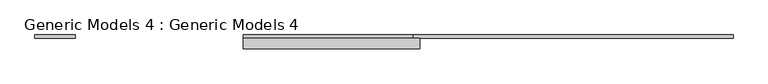
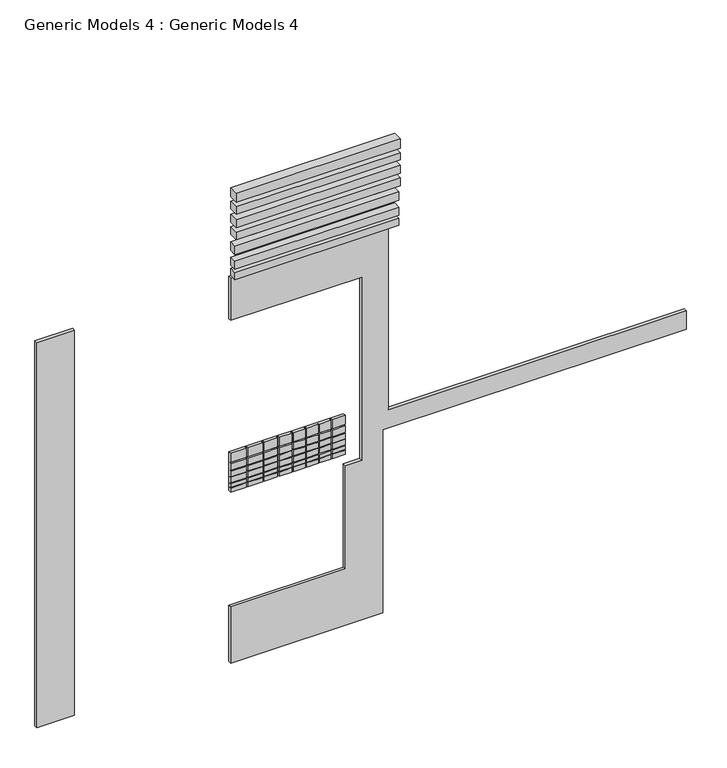
"""IFC4 building model written with IfcOpenShell, lengths in millimetres: proxy geometry, Generic Models 4 : Generic Models 4."""

from ifc_helpers import new_model, si_unit, frame, origin, origin_with_axes, place, context, project, spatial, polyline, outline, extrude, faceted_brep, source, transform, mapped, element, save


def generic_models_4_generic_models_4_7ccdd1b4(model_context):
    return source(origin(), model_context, "Body", "SolidModel", [
        faceted_brep([(-14590.3624893, -13038.0040375, 3489.9238444), (-14590.3624893, -13038.0040375, 3343.084444), (-14347.53389, -13038.0040375, 3343.084444), (-14347.53389, -13038.0040375, 3489.9238444), (-14590.3624893, -13038.0040375, 3318.5039332), (-14590.3624893, -13038.0040375, 3211.3169884), (-14347.53389, -13038.0040375, 3211.3169884), (-14347.53389, -13038.0040375, 3318.5039332), (-14590.3624893, -13038.0040375, 3195.0457498), (-14590.3624893, -13038.0040375, 3104.1608837), (-14347.53389, -13038.0040375, 3104.1608837), (-14347.53389, -13038.0040375, 3195.0457498), (-14590.3624893, -13038.0040375, 3090.4767451), (-14590.3624893, -13038.0040375, 3001.9466793), (-14347.53389, -13038.0040375, 3001.9466793), (-14347.53389, -13038.0040375, 3090.4767451), (-14590.3624893, -13038.0040375, 2913.8921657), (-14590.3624893, -13038.0040375, 2844.1911654), (-14347.53389, -13038.0040375, 2844.1911654), (-14347.53389, -13038.0040375, 2913.8921657), (-14590.3624893, -13038.0040375, 2982.1939105), (-14590.3624893, -13038.0040375, 2924.0827754), (-14347.53389, -13038.0040375, 2924.0827754), (-14347.53389, -13038.0040375, 2982.1939105), (-12786.9624893, -13038.0040375, 3343.084444), (-12786.9624893, -13038.0040375, 3489.9238444), (-12995.2571211, -13038.0040375, 3489.9238444), (-12995.2571211, -13038.0040375, 3343.084444), (-12786.9624893, -13038.0040375, 3211.3169884), (-12786.9624893, -13038.0040375, 3318.5039332), (-12995.2571211, -13038.0040375, 3318.5039332), (-12995.2571211, -13038.0040375, 3211.3169884), (-12786.9624893, -13038.0040375, 3104.1608837), (-12786.9624893, -13038.0040375, 3195.0457498), (-12995.2571211, -13038.0040375, 3195.0457498), (-12995.2571211, -13038.0040375, 3104.1608837), (-12786.9624893, -13038.0040375, 3001.9466793), (-12786.9624893, -13038.0040375, 3090.4767451), (-12995.2571211, -13038.0040375, 3090.4767451), (-12995.2571211, -13038.0040375, 3001.9466793), (-12786.9624893, -13038.0040375, 2844.1911654), (-12786.9624893, -13038.0040375, 2913.8921657), (-12995.2571211, -13038.0040375, 2913.8921657), (-12995.2571211, -13038.0040375, 2844.1911654), (-12786.9624893, -13038.0040375, 2924.0827754), (-12786.9624893, -13038.0040375, 2982.1939105), (-12995.2571211, -13038.0040375, 2982.1939105), (-12995.2571211, -13038.0040375, 2924.0827754), (-14088.2664986, -13038.0040375, 3489.9238444), (-14322.8470493, -13038.0040375, 3489.9238444), (-14322.8470493, -13038.0040375, 3343.084444), (-14088.2664986, -13038.0040375, 3343.084444), (-13853.6859479, -13038.0040375, 3489.9238444), (-14061.0687536, -13038.0040375, 3489.9238444), (-14061.0687536, -13038.0040375, 3343.084444), (-13853.6859479, -13038.0040375, 3343.084444), (-13632.7042697, -13038.0040375, 3489.9238444), (-13828.188062, -13038.0040375, 3489.9238444), (-13828.188062, -13038.0040375, 3343.084444), (-13632.7042697, -13038.0040375, 3343.084444), (-13419.8458226, -13038.0040375, 3489.9238444), (-13605.5065247, -13038.0040375, 3489.9238444), (-13605.5065247, -13038.0040375, 3343.084444), (-13419.8458226, -13038.0040375, 3343.084444), (-13214.5389402, -13038.0040375, 3489.9238444), (-13391.3242828, -13038.0040375, 3489.9238444), (-13391.3242828, -13038.0040375, 3343.084444), (-13214.5389402, -13038.0040375, 3343.084444), (-13013.9555708, -13038.0040375, 3489.9238444), (-13197.5403496, -13038.0040375, 3489.9238444), (-13197.5403496, -13038.0040375, 3343.084444), (-13013.9555708, -13038.0040375, 3343.084444), (-14322.8470493, -13038.0040375, 2844.1911654), (-14088.2664986, -13038.0040375, 2844.1911654), (-14088.2664986, -13038.0040375, 2913.8921657), (-14322.8470493, -13038.0040375, 2913.8921657), (-14061.0687536, -13038.0040375, 2844.1911654), (-13853.6859479, -13038.0040375, 2844.1911654), (-13853.6859479, -13038.0040375, 2913.8921657), (-14061.0687536, -13038.0040375, 2913.8921657), (-13828.188062, -13038.0040375, 2844.1911654), (-13632.7042697, -13038.0040375, 2844.1911654), (-13632.7042697, -13038.0040375, 2913.8921657), (-13828.188062, -13038.0040375, 2913.8921657), (-13605.5065247, -13038.0040375, 2844.1911654), (-13419.8458226, -13038.0040375, 2844.1911654), (-13419.8458226, -13038.0040375, 2913.8921657), (-13605.5065247, -13038.0040375, 2913.8921657), (-13391.3242828, -13038.0040375, 2844.1911654), (-13214.5389402, -13038.0040375, 2844.1911654), (-13214.5389402, -13038.0040375, 2913.8921657), (-13391.3242828, -13038.0040375, 2913.8921657), (-13197.5403496, -13038.0040375, 2844.1911654), (-13013.9555708, -13038.0040375, 2844.1911654), (-13013.9555708, -13038.0040375, 2913.8921657), (-13197.5403496, -13038.0040375, 2913.8921657), (-14322.8470493, -13038.0040375, 3211.3169884), (-14088.2664986, -13038.0040375, 3211.3169884), (-14088.2664986, -13038.0040375, 3318.5039332), (-14322.8470493, -13038.0040375, 3318.5039332), (-14061.0687536, -13038.0040375, 3211.3169884), (-13853.6859479, -13038.0040375, 3211.3169884), (-13853.6859479, -13038.0040375, 3318.5039332), (-14061.0687536, -13038.0040375, 3318.5039332), (-13828.188062, -13038.0040375, 3211.3169884), (-13632.7042697, -13038.0040375, 3211.3169884), (-13632.7042697, -13038.0040375, 3318.5039332), (-13828.188062, -13038.0040375, 3318.5039332), (-13605.5065247, -13038.0040375, 3211.3169884), (-13419.8458226, -13038.0040375, 3211.3169884), (-13419.8458226, -13038.0040375, 3318.5039332), (-13605.5065247, -13038.0040375, 3318.5039332), (-13391.3242828, -13038.0040375, 3211.3169884), (-13214.5389402, -13038.0040375, 3211.3169884), (-13214.5389402, -13038.0040375, 3318.5039332), (-13391.3242828, -13038.0040375, 3318.5039332), (-13197.5403496, -13038.0040375, 3211.3169884), (-13013.9555708, -13038.0040375, 3211.3169884), (-13013.9555708, -13038.0040375, 3318.5039332), (-13197.5403496, -13038.0040375, 3318.5039332), (-14322.8470493, -13038.0040375, 3104.1608837), (-14088.2664986, -13038.0040375, 3104.1608837), (-14088.2664986, -13038.0040375, 3195.0457498), (-14322.8470493, -13038.0040375, 3195.0457498), (-14061.0687536, -13038.0040375, 3104.1608837), (-13853.6859479, -13038.0040375, 3104.1608837), (-13853.6859479, -13038.0040375, 3195.0457498), (-14061.0687536, -13038.0040375, 3195.0457498), (-13828.188062, -13038.0040375, 3104.1608837), (-13632.7042697, -13038.0040375, 3104.1608837), (-13632.7042697, -13038.0040375, 3195.0457498), (-13828.188062, -13038.0040375, 3195.0457498), (-13605.5065247, -13038.0040375, 3104.1608837), (-13419.8458226, -13038.0040375, 3104.1608837), (-13419.8458226, -13038.0040375, 3195.0457498), (-13605.5065247, -13038.0040375, 3195.0457498), (-13391.3242828, -13038.0040375, 3104.1608837), (-13214.5389402, -13038.0040375, 3104.1608837), (-13214.5389402, -13038.0040375, 3195.0457498), (-13391.3242828, -13038.0040375, 3195.0457498), (-13197.5403496, -13038.0040375, 3104.1608837), (-13013.9555708, -13038.0040375, 3104.1608837), (-13013.9555708, -13038.0040375, 3195.0457498), (-13197.5403496, -13038.0040375, 3195.0457498), (-14322.8470493, -13038.0040375, 3001.9466793), (-14088.2664986, -13038.0040375, 3001.9466793), (-14088.2664986, -13038.0040375, 3090.4767451), (-14322.8470493, -13038.0040375, 3090.4767451), (-14061.0687536, -13038.0040375, 3001.9466793), (-13853.6859479, -13038.0040375, 3001.9466793), (-13853.6859479, -13038.0040375, 3090.4767451), (-14061.0687536, -13038.0040375, 3090.4767451), (-13828.188062, -13038.0040375, 3001.9466793), (-13632.7042697, -13038.0040375, 3001.9466793), (-13632.7042697, -13038.0040375, 3090.4767451), (-13828.188062, -13038.0040375, 3090.4767451), (-13605.5065247, -13038.0040375, 3001.9466793), (-13419.8458226, -13038.0040375, 3001.9466793), (-13419.8458226, -13038.0040375, 3090.4767451), (-13605.5065247, -13038.0040375, 3090.4767451), (-13391.3242828, -13038.0040375, 3001.9466793), (-13214.5389402, -13038.0040375, 3001.9466793), (-13214.5389402, -13038.0040375, 3090.4767451), (-13391.3242828, -13038.0040375, 3090.4767451), (-13197.5403496, -13038.0040375, 3001.9466793), (-13013.9555708, -13038.0040375, 3001.9466793), (-13013.9555708, -13038.0040375, 3090.4767451), (-13197.5403496, -13038.0040375, 3090.4767451), (-14322.8470493, -13038.0040375, 2924.0827754), (-14088.2664986, -13038.0040375, 2924.0827754), (-14088.2664986, -13038.0040375, 2982.1939105), (-14322.8470493, -13038.0040375, 2982.1939105), (-14061.0687536, -13038.0040375, 2924.0827754), (-13853.6859479, -13038.0040375, 2924.0827754), (-13853.6859479, -13038.0040375, 2982.1939105), (-14061.0687536, -13038.0040375, 2982.1939105), (-13828.188062, -13038.0040375, 2924.0827754), (-13632.7042697, -13038.0040375, 2924.0827754), (-13632.7042697, -13038.0040375, 2982.1939105), (-13828.188062, -13038.0040375, 2982.1939105), (-13605.5065247, -13038.0040375, 2924.0827754), (-13419.8458226, -13038.0040375, 2924.0827754), (-13419.8458226, -13038.0040375, 2982.1939105), (-13605.5065247, -13038.0040375, 2982.1939105), (-13391.3242828, -13038.0040375, 2924.0827754), (-13214.5389402, -13038.0040375, 2924.0827754), (-13214.5389402, -13038.0040375, 2982.1939105), (-13391.3242828, -13038.0040375, 2982.1939105), (-13197.5403496, -13038.0040375, 2924.0827754), (-13013.9555708, -13038.0040375, 2924.0827754), (-13013.9555708, -13038.0040375, 2982.1939105), (-13197.5403496, -13038.0040375, 2982.1939105), (-12786.9624893, -12987.2040375, 3489.9238444), (-12786.9624893, -12987.2040375, 2844.1911654), (-14590.3624893, -12987.2040375, 2844.1911654), (-14590.3624893, -12987.2040375, 3489.9238444), (-14347.53389, -13012.6040375, 3489.9238444), (-14322.8470493, -13012.6040375, 3489.9238444), (-14088.2664986, -13012.6040375, 3489.9238444), (-14061.0687536, -13012.6040375, 3489.9238444), (-13853.6859479, -13012.6040375, 3489.9238444), (-13828.188062, -13012.6040375, 3489.9238444), (-13632.7042697, -13012.6040375, 3489.9238444), (-13605.5065247, -13012.6040375, 3489.9238444), (-13419.8458226, -13012.6040375, 3489.9238444), (-13391.3242828, -13012.6040375, 3489.9238444), (-13214.5389402, -13012.6040375, 3489.9238444), (-13197.5403496, -13012.6040375, 3489.9238444), (-13013.9555708, -13012.6040375, 3489.9238444), (-12995.2571211, -13012.6040375, 3489.9238444), (-14590.3624893, -13012.6040375, 2913.8921657), (-14590.3624893, -13012.6040375, 2924.0827754), (-14590.3624893, -13012.6040375, 2982.1939105), (-14590.3624893, -13012.6040375, 3001.9466793), (-14590.3624893, -13012.6040375, 3090.4767451), (-14590.3624893, -13012.6040375, 3104.1608837), (-14590.3624893, -13012.6040375, 3195.0457498), (-14590.3624893, -13012.6040375, 3211.3169884), (-14590.3624893, -13012.6040375, 3318.5039332), (-14590.3624893, -13012.6040375, 3343.084444), (-12995.2571211, -13012.6040375, 2844.1911654), (-13013.9555708, -13012.6040375, 2844.1911654), (-13197.5403496, -13012.6040375, 2844.1911654), (-13214.5389402, -13012.6040375, 2844.1911654), (-13391.3242828, -13012.6040375, 2844.1911654), (-13419.8458226, -13012.6040375, 2844.1911654), (-13605.5065247, -13012.6040375, 2844.1911654), (-13632.7042697, -13012.6040375, 2844.1911654), (-13828.188062, -13012.6040375, 2844.1911654), (-13853.6859479, -13012.6040375, 2844.1911654), (-14061.0687536, -13012.6040375, 2844.1911654), (-14088.2664986, -13012.6040375, 2844.1911654), (-14322.8470493, -13012.6040375, 2844.1911654), (-14347.53389, -13012.6040375, 2844.1911654), (-12786.9624893, -13012.6040375, 3343.084444), (-12786.9624893, -13012.6040375, 3318.5039332), (-12786.9624893, -13012.6040375, 3211.3169884), (-12786.9624893, -13012.6040375, 3195.0457498), (-12786.9624893, -13012.6040375, 3104.1608837), (-12786.9624893, -13012.6040375, 3090.4767451), (-12786.9624893, -13012.6040375, 3001.9466793), (-12786.9624893, -13012.6040375, 2982.1939105), (-12786.9624893, -13012.6040375, 2924.0827754), (-12786.9624893, -13012.6040375, 2913.8921657), (-14347.53389, -13012.6040375, 3318.5039332), (-14347.53389, -13012.6040375, 3211.3169884), (-14347.53389, -13012.6040375, 3195.0457498), (-14347.53389, -13012.6040375, 3104.1608837), (-14347.53389, -13012.6040375, 3090.4767451), (-14347.53389, -13012.6040375, 3001.9466793), (-14347.53389, -13012.6040375, 2982.1939105), (-14347.53389, -13012.6040375, 2924.0827754), (-14347.53389, -13012.6040375, 2913.8921657), (-14322.8470493, -13012.6040375, 2913.8921657), (-14088.2664986, -13012.6040375, 2913.8921657), (-14061.0687536, -13012.6040375, 2913.8921657), (-13853.6859479, -13012.6040375, 2913.8921657), (-13828.188062, -13012.6040375, 2913.8921657), (-13632.7042697, -13012.6040375, 2913.8921657), (-13605.5065247, -13012.6040375, 2913.8921657), (-13419.8458226, -13012.6040375, 2913.8921657), (-13391.3242828, -13012.6040375, 2913.8921657), (-13214.5389402, -13012.6040375, 2913.8921657), (-13197.5403496, -13012.6040375, 2913.8921657), (-13013.9555708, -13012.6040375, 2913.8921657), (-12995.2571211, -13012.6040375, 2913.8921657), (-12995.2571211, -13012.6040375, 2924.0827754), (-12995.2571211, -13012.6040375, 2982.1939105), (-12995.2571211, -13012.6040375, 3001.9466793), (-12995.2571211, -13012.6040375, 3090.4767451), (-12995.2571211, -13012.6040375, 3104.1608837), (-12995.2571211, -13012.6040375, 3195.0457498), (-12995.2571211, -13012.6040375, 3211.3169884), (-12995.2571211, -13012.6040375, 3318.5039332), (-12995.2571211, -13012.6040375, 3343.084444), (-13013.9555708, -13012.6040375, 3343.084444), (-13197.5403496, -13012.6040375, 3343.084444), (-13214.5389402, -13012.6040375, 3343.084444), (-13391.3242828, -13012.6040375, 3343.084444), (-13419.8458226, -13012.6040375, 3343.084444), (-13605.5065247, -13012.6040375, 3343.084444), (-13632.7042697, -13012.6040375, 3343.084444), (-13828.188062, -13012.6040375, 3343.084444), (-13853.6859479, -13012.6040375, 3343.084444), (-14061.0687536, -13012.6040375, 3343.084444), (-14088.2664986, -13012.6040375, 3343.084444), (-14322.8470493, -13012.6040375, 3343.084444), (-14347.53389, -13012.6040375, 3343.084444), (-14322.8470493, -13012.6040375, 3318.5039332), (-14088.2664986, -13012.6040375, 3318.5039332), (-14088.2664986, -13012.6040375, 3211.3169884), (-14322.8470493, -13012.6040375, 3211.3169884), (-14061.0687536, -13012.6040375, 3318.5039332), (-13853.6859479, -13012.6040375, 3318.5039332), (-13853.6859479, -13012.6040375, 3211.3169884), (-14061.0687536, -13012.6040375, 3211.3169884), (-13828.188062, -13012.6040375, 3318.5039332), (-13632.7042697, -13012.6040375, 3318.5039332), (-13632.7042697, -13012.6040375, 3211.3169884), (-13828.188062, -13012.6040375, 3211.3169884), (-13605.5065247, -13012.6040375, 3318.5039332), (-13419.8458226, -13012.6040375, 3318.5039332), (-13419.8458226, -13012.6040375, 3211.3169884), (-13605.5065247, -13012.6040375, 3211.3169884), (-13391.3242828, -13012.6040375, 3318.5039332), (-13214.5389402, -13012.6040375, 3318.5039332), (-13214.5389402, -13012.6040375, 3211.3169884), (-13391.3242828, -13012.6040375, 3211.3169884), (-13197.5403496, -13012.6040375, 3318.5039332), (-13013.9555708, -13012.6040375, 3318.5039332), (-13013.9555708, -13012.6040375, 3211.3169884), (-13197.5403496, -13012.6040375, 3211.3169884), (-14322.8470493, -13012.6040375, 3195.0457498), (-14088.2664986, -13012.6040375, 3195.0457498), (-14088.2664986, -13012.6040375, 3104.1608837), (-14322.8470493, -13012.6040375, 3104.1608837), (-14061.0687536, -13012.6040375, 3195.0457498), (-13853.6859479, -13012.6040375, 3195.0457498), (-13853.6859479, -13012.6040375, 3104.1608837), (-14061.0687536, -13012.6040375, 3104.1608837), (-13828.188062, -13012.6040375, 3195.0457498), (-13632.7042697, -13012.6040375, 3195.0457498), (-13632.7042697, -13012.6040375, 3104.1608837), (-13828.188062, -13012.6040375, 3104.1608837), (-13605.5065247, -13012.6040375, 3195.0457498), (-13419.8458226, -13012.6040375, 3195.0457498), (-13419.8458226, -13012.6040375, 3104.1608837), (-13605.5065247, -13012.6040375, 3104.1608837), (-13391.3242828, -13012.6040375, 3195.0457498), (-13214.5389402, -13012.6040375, 3195.0457498), (-13214.5389402, -13012.6040375, 3104.1608837), (-13391.3242828, -13012.6040375, 3104.1608837), (-13197.5403496, -13012.6040375, 3195.0457498), (-13013.9555708, -13012.6040375, 3195.0457498), (-13013.9555708, -13012.6040375, 3104.1608837), (-13197.5403496, -13012.6040375, 3104.1608837), (-14322.8470493, -13012.6040375, 3090.4767451), (-14088.2664986, -13012.6040375, 3090.4767451), (-14088.2664986, -13012.6040375, 3001.9466793), (-14322.8470493, -13012.6040375, 3001.9466793), (-14061.0687536, -13012.6040375, 3090.4767451), (-13853.6859479, -13012.6040375, 3090.4767451), (-13853.6859479, -13012.6040375, 3001.9466793), (-14061.0687536, -13012.6040375, 3001.9466793), (-13828.188062, -13012.6040375, 3090.4767451), (-13632.7042697, -13012.6040375, 3090.4767451), (-13632.7042697, -13012.6040375, 3001.9466793), (-13828.188062, -13012.6040375, 3001.9466793), (-13605.5065247, -13012.6040375, 3090.4767451), (-13419.8458226, -13012.6040375, 3090.4767451), (-13419.8458226, -13012.6040375, 3001.9466793), (-13605.5065247, -13012.6040375, 3001.9466793), (-13391.3242828, -13012.6040375, 3090.4767451), (-13214.5389402, -13012.6040375, 3090.4767451), (-13214.5389402, -13012.6040375, 3001.9466793), (-13391.3242828, -13012.6040375, 3001.9466793), (-13197.5403496, -13012.6040375, 3090.4767451), (-13013.9555708, -13012.6040375, 3090.4767451), (-13013.9555708, -13012.6040375, 3001.9466793), (-13197.5403496, -13012.6040375, 3001.9466793), (-14322.8470493, -13012.6040375, 2982.1939105), (-14088.2664986, -13012.6040375, 2982.1939105), (-14088.2664986, -13012.6040375, 2924.0827754), (-14322.8470493, -13012.6040375, 2924.0827754), (-14061.0687536, -13012.6040375, 2982.1939105), (-13853.6859479, -13012.6040375, 2982.1939105), (-13853.6859479, -13012.6040375, 2924.0827754), (-14061.0687536, -13012.6040375, 2924.0827754), (-13828.188062, -13012.6040375, 2982.1939105), (-13632.7042697, -13012.6040375, 2982.1939105), (-13632.7042697, -13012.6040375, 2924.0827754), (-13828.188062, -13012.6040375, 2924.0827754), (-13605.5065247, -13012.6040375, 2982.1939105), (-13419.8458226, -13012.6040375, 2982.1939105), (-13419.8458226, -13012.6040375, 2924.0827754), (-13605.5065247, -13012.6040375, 2924.0827754), (-13391.3242828, -13012.6040375, 2982.1939105), (-13214.5389402, -13012.6040375, 2982.1939105), (-13214.5389402, -13012.6040375, 2924.0827754), (-13391.3242828, -13012.6040375, 2924.0827754), (-13197.5403496, -13012.6040375, 2982.1939105), (-13013.9555708, -13012.6040375, 2982.1939105), (-13013.9555708, -13012.6040375, 2924.0827754), (-13197.5403496, -13012.6040375, 2924.0827754)], [[[0, 1, 2, 3]], [[4, 5, 6, 7]], [[8, 9, 10, 11]], [[12, 13, 14, 15]], [[16, 17, 18, 19]], [[20, 21, 22, 23]], [[24, 25, 26, 27]], [[28, 29, 30, 31]], [[32, 33, 34, 35]], [[36, 37, 38, 39]], [[40, 41, 42, 43]], [[44, 45, 46, 47]], [[48, 49, 50, 51]], [[52, 53, 54, 55]], [[56, 57, 58, 59]], [[60, 61, 62, 63]], [[64, 65, 66, 67]], [[68, 69, 70, 71]], [[72, 73, 74, 75]], [[76, 77, 78, 79]], [[80, 81, 82, 83]], [[84, 85, 86, 87]], [[88, 89, 90, 91]], [[92, 93, 94, 95]], [[96, 97, 98, 99]], [[100, 101, 102, 103]], [[104, 105, 106, 107]], [[108, 109, 110, 111]], [[112, 113, 114, 115]], [[116, 117, 118, 119]], [[120, 121, 122, 123]], [[124, 125, 126, 127]], [[128, 129, 130, 131]], [[132, 133, 134, 135]], [[136, 137, 138, 139]], [[140, 141, 142, 143]], [[144, 145, 146, 147]], [[148, 149, 150, 151]], [[152, 153, 154, 155]], [[156, 157, 158, 159]], [[160, 161, 162, 163]], [[164, 165, 166, 167]], [[168, 169, 170, 171]], [[172, 173, 174, 175]], [[176, 177, 178, 179]], [[180, 181, 182, 183]], [[184, 185, 186, 187]], [[188, 189, 190, 191]], [[192, 193, 194, 195]], [[192, 195, 0, 3, 196, 197, 49, 48, 198, 199, 53, 52, 200, 201, 57, 56, 202, 203, 61, 60, 204, 205, 65, 64, 206, 207, 69, 68, 208, 209, 26, 25]], [[195, 194, 17, 16, 210, 211, 21, 20, 212, 213, 13, 12, 214, 215, 9, 8, 216, 217, 5, 4, 218, 219, 1, 0]], [[194, 193, 40, 43, 220, 221, 93, 92, 222, 223, 89, 88, 224, 225, 85, 84, 226, 227, 81, 80, 228, 229, 77, 76, 230, 231, 73, 72, 232, 233, 18, 17]], [[193, 192, 25, 24, 234, 235, 29, 28, 236, 237, 33, 32, 238, 239, 37, 36, 240, 241, 45, 44, 242, 243, 41, 40]], [[219, 218, 244, 245, 217, 216, 246, 247, 215, 214, 248, 249, 213, 212, 250, 251, 211, 210, 252, 233, 232, 253, 254, 231, 230, 255, 256, 229, 228, 257, 258, 227, 226, 259, 260, 225, 224, 261, 262, 223, 222, 263, 264, 221, 220, 265, 243, 242, 266, 267, 241, 240, 268, 269, 239, 238, 270, 271, 237, 236, 272, 273, 235, 234, 274, 209, 208, 275, 276, 207, 206, 277, 278, 205, 204, 279, 280, 203, 202, 281, 282, 201, 200, 283, 284, 199, 198, 285, 286, 197, 196, 287], [288, 289, 290, 291], [292, 293, 294, 295], [296, 297, 298, 299], [300, 301, 302, 303], [304, 305, 306, 307], [308, 309, 310, 311], [312, 313, 314, 315], [316, 317, 318, 319], [320, 321, 322, 323], [324, 325, 326, 327], [328, 329, 330, 331], [332, 333, 334, 335], [336, 337, 338, 339], [340, 341, 342, 343], [344, 345, 346, 347], [348, 349, 350, 351], [352, 353, 354, 355], [356, 357, 358, 359], [360, 361, 362, 363], [364, 365, 366, 367], [368, 369, 370, 371], [372, 373, 374, 375], [376, 377, 378, 379], [380, 381, 382, 383]], [[99, 98, 289, 288]], [[103, 102, 293, 292]], [[107, 106, 297, 296]], [[111, 110, 301, 300]], [[115, 114, 305, 304]], [[119, 118, 309, 308]], [[218, 4, 7, 244]], [[29, 235, 273, 30]], [[51, 50, 286, 285]], [[55, 54, 284, 283]], [[59, 58, 282, 281]], [[63, 62, 280, 279]], [[67, 66, 278, 277]], [[71, 70, 276, 275]], [[1, 219, 287, 2]], [[234, 24, 27, 274]], [[123, 122, 313, 312]], [[127, 126, 317, 316]], [[131, 130, 321, 320]], [[135, 134, 325, 324]], [[139, 138, 329, 328]], [[143, 142, 333, 332]], [[216, 8, 11, 246]], [[33, 237, 271, 34]], [[97, 96, 291, 290]], [[101, 100, 295, 294]], [[105, 104, 299, 298]], [[109, 108, 303, 302]], [[113, 112, 307, 306]], [[117, 116, 311, 310]], [[5, 217, 245, 6]], [[236, 28, 31, 272]], [[147, 146, 337, 336]], [[151, 150, 341, 340]], [[155, 154, 345, 344]], [[159, 158, 349, 348]], [[163, 162, 353, 352]], [[167, 166, 357, 356]], [[214, 12, 15, 248]], [[37, 239, 269, 38]], [[121, 120, 315, 314]], [[125, 124, 319, 318]], [[129, 128, 323, 322]], [[133, 132, 327, 326]], [[137, 136, 331, 330]], [[141, 140, 335, 334]], [[9, 215, 247, 10]], [[238, 32, 35, 270]], [[171, 170, 361, 360]], [[175, 174, 365, 364]], [[179, 178, 369, 368]], [[183, 182, 373, 372]], [[187, 186, 377, 376]], [[191, 190, 381, 380]], [[212, 20, 23, 250]], [[45, 241, 267, 46]], [[145, 144, 339, 338]], [[149, 148, 343, 342]], [[153, 152, 347, 346]], [[157, 156, 351, 350]], [[161, 160, 355, 354]], [[165, 164, 359, 358]], [[13, 213, 249, 14]], [[240, 36, 39, 268]], [[75, 74, 254, 253]], [[79, 78, 256, 255]], [[83, 82, 258, 257]], [[87, 86, 260, 259]], [[91, 90, 262, 261]], [[95, 94, 264, 263]], [[210, 16, 19, 252]], [[41, 243, 265, 42]], [[169, 168, 363, 362]], [[173, 172, 367, 366]], [[177, 176, 371, 370]], [[181, 180, 375, 374]], [[185, 184, 379, 378]], [[189, 188, 383, 382]], [[21, 211, 251, 22]], [[242, 44, 47, 266]], [[253, 232, 72, 75]], [[197, 286, 50, 49]], [[288, 291, 96, 99]], [[312, 315, 120, 123]], [[336, 339, 144, 147]], [[360, 363, 168, 171]], [[245, 244, 7, 6]], [[247, 246, 11, 10]], [[249, 248, 15, 14]], [[251, 250, 23, 22]], [[233, 252, 19, 18]], [[287, 196, 3, 2]], [[255, 230, 76, 79]], [[199, 284, 54, 53]], [[292, 295, 100, 103]], [[316, 319, 124, 127]], [[340, 343, 148, 151]], [[364, 367, 172, 175]], [[231, 254, 74, 73]], [[285, 198, 48, 51]], [[290, 289, 98, 97]], [[314, 313, 122, 121]], [[338, 337, 146, 145]], [[362, 361, 170, 169]], [[257, 228, 80, 83]], [[201, 282, 58, 57]], [[296, 299, 104, 107]], [[320, 323, 128, 131]], [[344, 347, 152, 155]], [[368, 371, 176, 179]], [[229, 256, 78, 77]], [[283, 200, 52, 55]], [[294, 293, 102, 101]], [[318, 317, 126, 125]], [[342, 341, 150, 149]], [[366, 365, 174, 173]], [[259, 226, 84, 87]], [[203, 280, 62, 61]], [[300, 303, 108, 111]], [[324, 327, 132, 135]], [[348, 351, 156, 159]], [[372, 375, 180, 183]], [[227, 258, 82, 81]], [[281, 202, 56, 59]], [[298, 297, 106, 105]], [[322, 321, 130, 129]], [[346, 345, 154, 153]], [[370, 369, 178, 177]], [[261, 224, 88, 91]], [[205, 278, 66, 65]], [[304, 307, 112, 115]], [[328, 331, 136, 139]], [[352, 355, 160, 163]], [[376, 379, 184, 187]], [[225, 260, 86, 85]], [[279, 204, 60, 63]], [[302, 301, 110, 109]], [[326, 325, 134, 133]], [[350, 349, 158, 157]], [[374, 373, 182, 181]], [[263, 222, 92, 95]], [[207, 276, 70, 69]], [[308, 311, 116, 119]], [[332, 335, 140, 143]], [[356, 359, 164, 167]], [[380, 383, 188, 191]], [[223, 262, 90, 89]], [[277, 206, 64, 67]], [[306, 305, 114, 113]], [[330, 329, 138, 137]], [[354, 353, 162, 161]], [[378, 377, 186, 185]], [[265, 220, 43, 42]], [[267, 266, 47, 46]], [[269, 268, 39, 38]], [[271, 270, 35, 34]], [[273, 272, 31, 30]], [[209, 274, 27, 26]], [[221, 264, 94, 93]], [[275, 208, 68, 71]], [[310, 309, 118, 117]], [[334, 333, 142, 141]], [[358, 357, 166, 165]], [[382, 381, 190, 189]]]),
        extrude(outline(polyline([(6400.8, -12113.8624893), (6400.8, -14590.3624893), (5700.0726993, -14590.3624893), (5700.0726993, -12530.5912799), (2655.984893, -12530.5912799), (2655.984893, -12786.9624893), (937.2723538, -12786.9624893), (937.2723538, -14590.3624893), (0.0, -14590.3624893), (0.0, -12194.0978368), (3048.0, -12194.0978368), (3048.0, -7427.5624893), (3352.8, -7427.5624893), (3352.8, -12113.8624893), (6400.8, -12113.8624893)])), frame((0.0, -13038.0040375, 0.0), z_axis=(0.0, 1.0, 0.0), x_axis=(0.0, 0.0, 1.0)), (0.0, 0.0, 1.0), 50.8),
        extrude(outline(polyline([(-17045.3354046, -13038.0040375), (-17638.3624893, -13038.0040375), (-17638.3624893, -12987.2040375), (-17045.3354046, -12987.2040375), (-17045.3354046, -13038.0040375)])), origin_with_axes(), (0.0, 0.0, 1.0), 6400.8),
        extrude(outline(polyline([(-12011.7257787, -13038.0040375), (-12011.7257787, -13190.4040375), (-14590.3624893, -13190.4040375), (-14590.3624893, -13038.0040375), (-12011.7257787, -13038.0040375)])), frame((0.0, 0.0, 7756.9291211), z_axis=(0.0, 0.0, 1.0), x_axis=(1.0, 0.0, 0.0)), (0.0, 0.0, 1.0), 152.4),
        extrude(outline(polyline([(-12011.7257787, -13038.0040375), (-12011.7257787, -13190.4040375), (-14590.3624893, -13190.4040375), (-14590.3624893, -13038.0040375), (-12011.7257787, -13038.0040375)])), frame((0.0, 0.0, 7560.0999778), z_axis=(0.0, 0.0, 1.0), x_axis=(1.0, 0.0, 0.0)), (0.0, 0.0, 1.0), 121.2038306),
        extrude(outline(polyline([(-12011.7257787, -13038.0040375), (-12011.7257787, -13190.4040375), (-14590.3624893, -13190.4040375), (-14590.3624893, -13038.0040375), (-12011.7257787, -13038.0040375)])), frame((0.0, 0.0, 7335.7249872), z_axis=(0.0, 0.0, 1.0), x_axis=(1.0, 0.0, 0.0)), (0.0, 0.0, 1.0), 132.4289587),
        extrude(outline(polyline([(-12011.7257787, -13038.0040375), (-12011.7257787, -13190.4040375), (-14590.3624893, -13190.4040375), (-14590.3624893, -13038.0040375), (-12011.7257787, -13038.0040375)])), frame((0.0, 0.0, 7132.5850888), z_axis=(0.0, 0.0, 1.0), x_axis=(1.0, 0.0, 0.0)), (0.0, 0.0, 1.0), 129.3507787),
        extrude(outline(polyline([(-12011.7257787, -13038.0040375), (-12011.7257787, -13156.1130831), (-14590.3624893, -13156.1130831), (-14590.3624893, -13038.0040375), (-12011.7257787, -13038.0040375)])), frame((0.0, 0.0, 6867.2855004), z_axis=(0.0, 0.0, 1.0), x_axis=(1.0, 0.0, 0.0)), (0.0, 0.0, 1.0), 139.253935),
        extrude(outline(polyline([(-12011.7257787, -13038.0040375), (-12011.7257787, -13156.1130831), (-14590.3624893, -13156.1130831), (-14590.3624893, -13038.0040375), (-12011.7257787, -13038.0040375)])), frame((0.0, 0.0, 6621.8242216), z_axis=(0.0, 0.0, 1.0), x_axis=(1.0, 0.0, 0.0)), (0.0, 0.0, 1.0), 133.0965407),
        extrude(outline(polyline([(-12011.7257787, -13038.0040375), (-12011.7257787, -13156.1130831), (-14590.3624893, -13156.1130831), (-14590.3624893, -13038.0040375), (-12011.7257787, -13038.0040375)])), frame((0.0, 0.0, 6452.2943916), z_axis=(0.0, 0.0, 1.0), x_axis=(1.0, 0.0, 0.0)), (0.0, 0.0, 1.0), 113.6662014),
    ])


if __name__ == "__main__":
    model = new_model("IFC4")
    model_context = context("Model", 3, world=origin())
    ifc_project = project(units=[si_unit("LENGTHUNIT", "METRE", prefix="MILLI")], contexts=[model_context])
    site = spatial("IfcSite", under=ifc_project)
    building = spatial("IfcBuilding", under=site)
    placement = place(None, origin())
    generic_models_4_generic_models_4_shape = generic_models_4_generic_models_4_7ccdd1b4(model_context)
    element("IfcBuildingElementProxy", 1, Name="Generic Models 4 : Generic Models 4", ObjectType="Generic Models 4 : Generic Models 4", at=placement, inside=building, context=model_context, shape_type="MappedRepresentation", body=[
        mapped(generic_models_4_generic_models_4_shape, transform((0.0, 0.0, 0.0), x_axis=(1.0, 0.0, 0.0), y_axis=(0.0, 1.0, 0.0), z_axis=(0.0, 0.0, 1.0))),
    ])
    save(model, "model.ifc")
